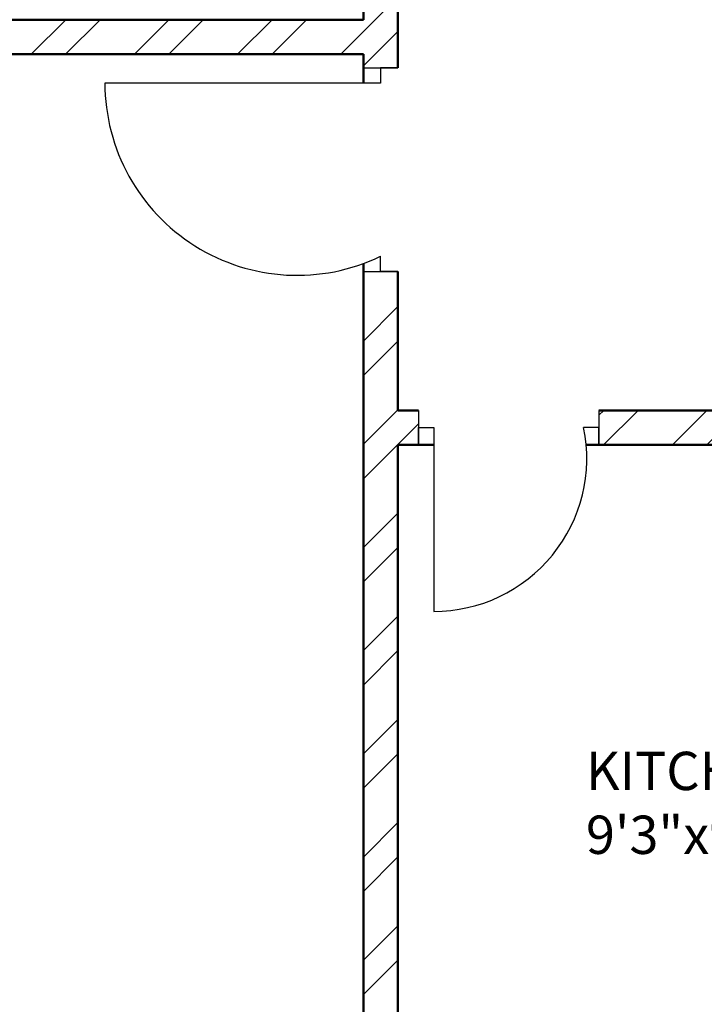
# Model space of a CAD drawing. Units: inches. Extents: x 963 to 2075, y 289 to 2657.
# Tile 44 of 98: x 1600 to 1689, y 1585 to 1714. Entities that reach past the tile are written whole.
import ezdxf

# ---------------------------------------------------------------- set-up
doc = ezdxf.new("R2010")
doc.units = ezdxf.units.IN
for name, color, linetype, lineweight in [('A-AREA-IDEN', 7, 'Continuous', 18), ('A-DOOR', 4, 'Continuous', 25), ('A-WALL', 7, 'Continuous', 50), ('A-WALL-PATT', 8, 'Continuous', 13)]:
    doc.layers.add(name, color=color, linetype=linetype, lineweight=lineweight)
doc.styles.get("Standard").update_dxf_attribs({"font": 'arial.ttf'})

msp = doc.modelspace()

# ---------------------------------------------------------------- hatches: boundary and pattern name
at = {"layer": 'A-WALL-PATT'}
h = msp.add_hatch(dxfattribs=at)
h.set_pattern_fill('ANSI32', color=256)
h.paths.add_polyline_path([(1296.92, 2558.32), (1203.92, 2558.32), (1203.92, 2493.82), (1191.53, 2493.82), (1191.53, 2489.32), (1211.06, 2489.32), (1211.06, 2492.02), (1211.06, 2493.82), (1208.42, 2493.82), (1208.42, 2553.82), (1292.42, 2553.82), (1292.42, 2538.86), (1296.92, 2538.86)])
h.paths.add_polyline_path([(1442.42, 2558.32), (1349.42, 2558.32), (1349.42, 2538.94), (1353.92, 2538.94), (1353.92, 2553.82), (1437.92, 2553.82), (1437.92, 2493.82), (1434.54, 2493.82), (1434.54, 2489.32), (1448.31, 2489.32), (1448.31, 2491.57), (1448.31, 2493.82), (1442.42, 2493.82)])
h.paths.add_polyline_path([(1415.55, 2491.57), (1415.55, 2493.82), (1340.94, 2493.82), (1340.94, 2489.32), (1371.92, 2489.32), (1371.92, 2378.32), (1367.6, 2378.32), (1367.6, 2373.82), (1371.92, 2373.82), (1371.92, 2355.19), (1376.42, 2355.19), (1376.42, 2489.32), (1415.55, 2489.32)])
h.paths.add_polyline_path([(1304.94, 2491.57), (1304.94, 2493.82), (1296.92, 2493.82), (1296.92, 2514.86), (1292.42, 2514.86), (1292.42, 2493.82), (1232.81, 2493.82), (1232.81, 2489.32), (1256.42, 2489.32), (1256.42, 2327.32), (1253.71, 2327.32), (1253.71, 2322.82), (1328.42, 2322.82), (1328.42, 2331.15), (1323.92, 2331.15), (1323.92, 2327.32), (1260.92, 2327.32), (1260.92, 2373.82), (1323.92, 2373.82), (1323.92, 2357.81), (1328.42, 2357.81), (1328.42, 2373.82), (1346.01, 2373.82), (1346.01, 2376.07), (1346.01, 2378.32), (1260.92, 2378.32), (1260.92, 2489.32), (1304.94, 2489.32)])
h.paths.add_polyline_path([(1226.65, 2327.32), (1124.42, 2327.32), (1124.42, 2347.45), (1119.92, 2347.45), (1119.92, 2322.82), (1163.42, 2322.82), (1163.42, 2305.43), (1165.67, 2305.43), (1167.92, 2305.43), (1167.92, 2322.82), (1226.65, 2322.82), (1226.65, 2325.07)])
h.paths.add_polyline_path([(1095.92, 2489.32), (1124.42, 2489.32), (1131.53, 2489.32), (1131.53, 2491.57), (1131.53, 2493.82), (1119.92, 2493.82), (1091.42, 2493.82), (1091.42, 2417.32), (1095.92, 2417.32), (1119.92, 2417.32), (1119.92, 2407.45), (1124.42, 2407.45), (1124.42, 2421.82), (1095.92, 2421.82)])
h.paths.add_polyline_path([(1512.92, 2558.32), (1508.42, 2558.32), (1508.42, 2493.82), (1503.4, 2493.82), (1503.4, 2489.32), (1508.42, 2489.32), (1508.42, 2327.32), (1376.42, 2327.32), (1376.42, 2330.27), (1371.92, 2330.27), (1371.92, 2298.74), (1376.42, 2298.74), (1376.42, 2322.82), (1508.42, 2322.82), (1508.42, 2165.32), (1504.26, 2165.32), (1504.26, 2160.82), (1508.42, 2160.82), (1508.42, 2108.32), (1512.92, 2108.32), (1512.92, 2160.82), (1516.18, 2160.82), (1516.18, 2163.07), (1516.18, 2165.32), (1512.92, 2165.32), (1512.92, 2322.82), (1644.92, 2322.82), (1644.92, 2298.74), (1649.42, 2298.74), (1649.42, 2322.82), (1649.42, 2330.94), (1647.17, 2330.94), (1644.92, 2330.94), (1644.92, 2327.32), (1512.92, 2327.32), (1512.92, 2489.32), (1516.76, 2489.32), (1516.76, 2491.57), (1516.76, 2493.82), (1512.92, 2493.82)])
h.paths.add_polyline_path([(1671.92, 2558.32), (1578.92, 2558.32), (1578.92, 2493.82), (1573.53, 2493.82), (1573.53, 2489.32), (1586.54, 2489.32), (1586.54, 2491.57), (1586.54, 2493.82), (1583.42, 2493.82), (1583.42, 2553.82), (1667.42, 2553.82), (1667.42, 2541.11), (1671.92, 2541.11)])
h.paths.add_polyline_path([(1681.26, 2493.82), (1671.92, 2493.82), (1671.92, 2517.11), (1667.42, 2517.11), (1667.42, 2493.82), (1610.22, 2493.82), (1610.22, 2489.32), (1644.92, 2489.32), (1644.92, 2357.87), (1649.42, 2357.87), (1649.42, 2373.82), (1652.2, 2373.82), (1652.2, 2375.83), (1652.2, 2378.32), (1649.42, 2378.32), (1649.42, 2489.32), (1681.26, 2489.32), (1681.26, 2491.57)])
h.paths.add_polyline_path([(1821.92, 2558.32), (1728.92, 2558.32), (1728.92, 2541), (1733.42, 2541), (1733.42, 2553.82), (1817.42, 2553.82), (1817.42, 2493.82), (1813.51, 2493.82), (1813.51, 2489.32), (1830.08, 2489.32), (1830.08, 2491.57), (1830.08, 2493.82), (1821.92, 2493.82)])
h.paths.add_polyline_path([(1794.24, 2493.82), (1717.26, 2493.82), (1717.26, 2489.32), (1760.42, 2489.32), (1760.42, 2378.32), (1674.4, 2378.32), (1674.4, 2373.82), (1692.92, 2373.82), (1692.92, 2356.95), (1697.42, 2356.95), (1697.42, 2373.82), (1760.42, 2373.82), (1760.42, 2327.32), (1697.42, 2327.32), (1697.42, 2333.34), (1692.92, 2333.34), (1692.92, 2322.82), (1768.04, 2322.82), (1768.04, 2325.07), (1768.04, 2327.32), (1764.92, 2327.32), (1764.92, 2489.32), (1794.24, 2489.32)])
h.paths.add_polyline_path([(1733.42, 2517), (1728.92, 2517), (1728.92, 2493.82), (1733.42, 2493.82)], flags=17)
h.paths.add_polyline_path([(1929.92, 2493.82), (1890.08, 2493.82), (1890.08, 2489.32), (1896.92, 2489.32), (1925.42, 2489.32), (1925.42, 2421.82), (1896.92, 2421.82), (1896.92, 2408.32), (1901.42, 2408.32), (1901.42, 2417.32), (1925.42, 2417.32), (1929.92, 2417.32)])
h.paths.add_polyline_path([(1901.42, 2348.32), (1896.92, 2348.32), (1896.92, 2327.32), (1800.42, 2327.32), (1800.42, 2322.82), (1853.42, 2322.82), (1853.42, 2309.45), (1857.92, 2309.45), (1857.92, 2322.82), (1901.42, 2322.82)])
h.paths.add_polyline_path([(1857.92, 2249.45), (1853.42, 2249.45), (1853.42, 2214.82), (1686.31, 2214.82), (1686.31, 2210.32), (1853.42, 2210.32), (1853.42, 2202.13), (1857.92, 2202.13), (1857.92, 2210.32)])
h.paths.add_polyline_path([(1857.92, 2142.13), (1853.42, 2142.13), (1853.42, 2115.42), (1841.42, 2115.42), (1841.42, 2088.53), (1841.42, 2046.95), (1845.92, 2046.95), (1845.92, 2110.92), (1905.92, 2110.92), (1905.92, 2092.52), (1910.42, 2092.52), (1910.42, 2115.42), (1857.92, 2115.42)])
h.paths.add_polyline_path([(1532.44, 1482.34), (1573.46, 1482.34), (1573.46, 1501), (1532.44, 1501)], flags=9)
h.paths.add_polyline_path([(1438.66, 1486.3), (1479.68, 1486.3), (1479.68, 1504.96), (1438.66, 1504.96)], flags=9)
h.paths.add_polyline_path([(1411.22, 1365.31), (1659.14, 1365.31), (1659.14, 1402.4), (1411.22, 1402.4)], flags=9)
h.paths.add_polyline_path([(1185.67, 2296.3), (1248.16, 2296.3), (1248.16, 2314.95), (1185.67, 2314.95)], flags=9)
h.paths.add_polyline_path([(1177.31, 2187.35), (1216.15, 2187.35), (1216.15, 2206.01), (1177.31, 2206.01)], flags=9)
h.paths.add_polyline_path([(1295.1, 1602.08), (1328.26, 1602.08), (1328.26, 1620.74), (1295.1, 1620.74)], flags=9)
h.paths.add_polyline_path([(1525.13, 2005.99), (1558.39, 2005.99), (1558.39, 2024.65), (1525.13, 2024.65)], flags=9)
h.paths.add_polyline_path([(1459.61, 1977.13), (1472.19, 1977.13), (1472.19, 1987.43), (1459.61, 1987.43)], flags=9)
h.paths.add_polyline_path([(1467.81, 2053.68), (1480.02, 2053.68), (1480.02, 2063.98), (1467.81, 2063.98)], flags=9)
h.paths.add_polyline_path([(1555.18, 2119.02), (1584.56, 2119.02), (1584.56, 2137.68), (1555.18, 2137.68)], flags=25)
h.paths.add_polyline_path([(1405.39, 2115.29), (1444.48, 2115.29), (1444.48, 2133.95), (1405.39, 2133.95)], flags=25)
h.paths.add_polyline_path([(1698.48, 2004.26), (1727.69, 2004.26), (1727.69, 2022.92), (1698.48, 2022.92)], flags=9)
h.paths.add_polyline_path([(1612.16, 1972.86), (1629.02, 1972.86), (1629.02, 1983.16), (1612.16, 1983.16)], flags=9)
h.paths.add_polyline_path([(1608.29, 2060.04), (1625.15, 2060.04), (1625.15, 2070.34), (1608.29, 2070.34)], flags=9)
h.paths.add_polyline_path([(1527.95, 1684.4), (1566.79, 1684.4), (1566.79, 1703.06), (1527.95, 1703.06)], flags=9)
h.paths.add_polyline_path([(1422.79, 1683.59), (1461.63, 1683.59), (1461.63, 1702.25), (1422.79, 1702.25)], flags=9)
h.paths.add_polyline_path([(1531.26, 1732.46), (1574.01, 1732.46), (1574.01, 1751.12), (1531.26, 1751.12)], flags=9)
h.paths.add_polyline_path([(1402.87, 1732.85), (1439.8, 1732.85), (1439.8, 1751.5), (1402.87, 1751.5)], flags=9)
h.paths.add_polyline_path([(1243.12, 1923.13), (1281.96, 1923.13), (1281.96, 1941.79), (1243.12, 1941.79)], flags=9)
h.paths.add_polyline_path([(1181.75, 1792.27), (1244.24, 1792.27), (1244.24, 1810.93), (1181.75, 1810.93)], flags=9)
h.paths.add_polyline_path([(1265.82, 1670.3), (1316.07, 1670.3), (1316.07, 1688.96), (1265.82, 1688.96)], flags=9)
h.paths.add_polyline_path([(1140.26, 1676.05), (1179.1, 1676.05), (1179.1, 1694.71), (1140.26, 1694.71)], flags=9)
h.paths.add_polyline_path([(1107.49, 1490.89), (1143.37, 1490.89), (1143.37, 1509.55), (1107.49, 1509.55)], flags=9)
h.paths.add_polyline_path([(1217.58, 1483.9), (1246.74, 1483.9), (1246.74, 1502.56), (1217.58, 1502.56)], flags=9)
h.paths.add_polyline_path([(1389.21, 1486.92), (1418.37, 1486.92), (1418.37, 1505.58), (1389.21, 1505.58)], flags=9)
h.paths.add_polyline_path([(1672.21, 1602.08), (1705.37, 1602.08), (1705.37, 1620.74), (1672.21, 1620.74)], flags=9)
h.paths.add_polyline_path([(1752.08, 1522.64), (1781.24, 1522.64), (1781.24, 1541.3), (1752.08, 1541.3)], flags=9)
h.paths.add_polyline_path([(1848.27, 1491.26), (1884.16, 1491.26), (1884.16, 1509.92), (1848.27, 1509.92)], flags=9)
h.paths.add_polyline_path([(1822.47, 1685.62), (1861.31, 1685.62), (1861.31, 1704.28), (1822.47, 1704.28)], flags=9)
h.paths.add_polyline_path([(1713.19, 1672.23), (1763.44, 1672.23), (1763.44, 1690.89), (1713.19, 1690.89)], flags=9)
h.paths.add_polyline_path([(1736.62, 1790.58), (1799.11, 1790.58), (1799.11, 1809.24), (1736.62, 1809.24)], flags=9)
h.paths.add_polyline_path([(1691.49, 1916.36), (1730.33, 1916.36), (1730.33, 1935.01), (1691.49, 1935.01)], flags=9)
h.paths.add_polyline_path([(1764.87, 1973.92), (1794.31, 1973.92), (1794.31, 1992.58), (1764.87, 1992.58)], flags=9)
h.paths.add_polyline_path([(1767.85, 2034.02), (1797.29, 2034.02), (1797.29, 2052.67), (1767.85, 2052.67)], flags=9)
h.paths.add_polyline_path([(1851.59, 2060.33), (1880.75, 2060.33), (1880.75, 2078.99), (1851.59, 2078.99)], flags=25)
h.paths.add_polyline_path([(1688.49, 2086.87), (1727.33, 2086.87), (1727.33, 2105.53), (1688.49, 2105.53)], flags=9)
h.paths.add_polyline_path([(1537.74, 2293.58), (1580.49, 2293.58), (1580.49, 2312.24), (1537.74, 2312.24)], flags=25)
h.paths.add_polyline_path([(1425.59, 2296.11), (1468.34, 2296.11), (1468.34, 2314.77), (1425.59, 2314.77)], flags=25)
h.paths.add_polyline_path([(1278.52, 2004.18), (1307.72, 2004.18), (1307.72, 2022.84), (1278.52, 2022.84)], flags=9)
h.paths.add_polyline_path([(1193.28, 1973.63), (1222.72, 1973.63), (1222.72, 1992.29), (1193.28, 1992.29)], flags=9)
h.paths.add_polyline_path([(1192.41, 2040.58), (1221.84, 2040.58), (1221.84, 2059.23), (1192.41, 2059.23)], flags=9)
h.paths.add_polyline_path([(1130.6, 1951.39), (1159.76, 1951.39), (1159.76, 1970.05), (1130.6, 1970.05)], flags=9)
h.paths.add_polyline_path([(1132.83, 2052.49), (1161.98, 2052.49), (1161.98, 2071.15), (1132.83, 2071.15)], flags=9)
h.paths.add_polyline_path([(1265.13, 2334.62), (1315.38, 2334.62), (1315.38, 2353.28), (1265.13, 2353.28)], flags=25)
h.paths.add_polyline_path([(1136.74, 2330.79), (1175.58, 2330.79), (1175.58, 2349.44), (1136.74, 2349.44)], flags=9)
h.paths.add_polyline_path([(1287.42, 2417.2), (1320.58, 2417.2), (1320.58, 2435.86), (1287.42, 2435.86)], flags=25)
h.paths.add_polyline_path([(1430.99, 2329.16), (1469.83, 2329.16), (1469.83, 2347.82), (1430.99, 2347.82)], flags=25)
h.paths.add_polyline_path([(1525.42, 2329.21), (1564.26, 2329.21), (1564.26, 2347.87), (1525.42, 2347.87)], flags=25)
h.paths.add_polyline_path([(1684.52, 2382.8), (1717.68, 2382.8), (1717.68, 2401.46), (1684.52, 2401.46)], flags=25)
h.paths.add_polyline_path([(1704.81, 2340.29), (1755.05, 2340.29), (1755.05, 2358.95), (1704.81, 2358.95)], flags=25)
h.paths.add_polyline_path([(1694.11, 2287.76), (1756.6, 2287.76), (1756.6, 2306.41), (1694.11, 2306.41)], flags=9)
h.paths.add_polyline_path([(1815.78, 2329.86), (1854.62, 2329.86), (1854.62, 2348.52), (1815.78, 2348.52)], flags=9)
h.paths.add_polyline_path([(1842.87, 2514.26), (1878.76, 2514.26), (1878.76, 2532.91), (1842.87, 2532.91)], flags=9)
h.paths.add_polyline_path([(1769.51, 2531.45), (1798.67, 2531.45), (1798.67, 2550.1), (1769.51, 2550.1)], flags=25)
h.paths.add_polyline_path([(1594.77, 2518.47), (1623.93, 2518.47), (1623.93, 2537.13), (1594.77, 2537.13)], flags=25)
h.paths.add_polyline_path([(1520.72, 2516.18), (1556.61, 2516.18), (1556.61, 2534.84), (1520.72, 2534.84)], flags=25)
h.paths.add_polyline_path([(1464.46, 2516.69), (1500.34, 2516.69), (1500.34, 2535.35), (1464.46, 2535.35)], flags=25)
h.paths.add_polyline_path([(1365.7, 2528.97), (1394.85, 2528.97), (1394.85, 2547.63), (1365.7, 2547.63)], flags=25)
h.paths.add_polyline_path([(1222.84, 2516.23), (1252, 2516.23), (1252, 2534.89), (1222.84, 2534.89)], flags=25)
h.paths.add_polyline_path([(1104.55, 2509.6), (1140.43, 2509.6), (1140.43, 2528.26), (1104.55, 2528.26)], flags=9)
h = msp.add_hatch(dxfattribs=at)
h.set_pattern_fill('ANSI32', color=256)
h.paths.add_polyline_path([(1335.97, 2212.57), (1335.97, 2214.82), (1167.92, 2214.82), (1167.92, 2245.43), (1163.42, 2245.43), (1163.42, 2210.32), (1163.42, 2194.81), (1167.92, 2194.81), (1167.92, 2210.32), (1335.97, 2210.32)])
h.paths.add_polyline_path([(1532.44, 1482.34), (1573.46, 1482.34), (1573.46, 1501), (1532.44, 1501)], flags=9)
h.paths.add_polyline_path([(1438.66, 1486.3), (1479.68, 1486.3), (1479.68, 1504.96), (1438.66, 1504.96)], flags=9)
h.paths.add_polyline_path([(1411.22, 1365.31), (1659.14, 1365.31), (1659.14, 1402.4), (1411.22, 1402.4)], flags=9)
h.paths.add_polyline_path([(1185.67, 2296.3), (1248.16, 2296.3), (1248.16, 2314.95), (1185.67, 2314.95)], flags=9)
h.paths.add_polyline_path([(1177.31, 2187.35), (1216.15, 2187.35), (1216.15, 2206.01), (1177.31, 2206.01)], flags=9)
h.paths.add_polyline_path([(1295.1, 1602.08), (1328.26, 1602.08), (1328.26, 1620.74), (1295.1, 1620.74)], flags=9)
h.paths.add_polyline_path([(1525.13, 2005.99), (1558.39, 2005.99), (1558.39, 2024.65), (1525.13, 2024.65)], flags=9)
h.paths.add_polyline_path([(1459.61, 1977.13), (1472.19, 1977.13), (1472.19, 1987.43), (1459.61, 1987.43)], flags=9)
h.paths.add_polyline_path([(1467.81, 2053.68), (1480.02, 2053.68), (1480.02, 2063.98), (1467.81, 2063.98)], flags=9)
h.paths.add_polyline_path([(1555.18, 2119.02), (1584.56, 2119.02), (1584.56, 2137.68), (1555.18, 2137.68)], flags=9)
h.paths.add_polyline_path([(1405.39, 2115.29), (1444.48, 2115.29), (1444.48, 2133.95), (1405.39, 2133.95)], flags=9)
h.paths.add_polyline_path([(1698.48, 2004.26), (1727.69, 2004.26), (1727.69, 2022.92), (1698.48, 2022.92)], flags=9)
h.paths.add_polyline_path([(1612.16, 1972.86), (1629.02, 1972.86), (1629.02, 1983.16), (1612.16, 1983.16)], flags=9)
h.paths.add_polyline_path([(1608.29, 2060.04), (1625.15, 2060.04), (1625.15, 2070.34), (1608.29, 2070.34)], flags=9)
h.paths.add_polyline_path([(1527.95, 1684.4), (1566.79, 1684.4), (1566.79, 1703.06), (1527.95, 1703.06)], flags=9)
h.paths.add_polyline_path([(1422.79, 1683.59), (1461.63, 1683.59), (1461.63, 1702.25), (1422.79, 1702.25)], flags=9)
h.paths.add_polyline_path([(1531.26, 1732.46), (1574.01, 1732.46), (1574.01, 1751.12), (1531.26, 1751.12)], flags=9)
h.paths.add_polyline_path([(1402.87, 1732.85), (1439.8, 1732.85), (1439.8, 1751.5), (1402.87, 1751.5)], flags=9)
h.paths.add_polyline_path([(1243.12, 1923.13), (1281.96, 1923.13), (1281.96, 1941.79), (1243.12, 1941.79)], flags=9)
h.paths.add_polyline_path([(1181.75, 1792.27), (1244.24, 1792.27), (1244.24, 1810.93), (1181.75, 1810.93)], flags=9)
h.paths.add_polyline_path([(1265.82, 1670.3), (1316.07, 1670.3), (1316.07, 1688.96), (1265.82, 1688.96)], flags=9)
h.paths.add_polyline_path([(1140.26, 1676.05), (1179.1, 1676.05), (1179.1, 1694.71), (1140.26, 1694.71)], flags=9)
h.paths.add_polyline_path([(1107.49, 1490.89), (1143.37, 1490.89), (1143.37, 1509.55), (1107.49, 1509.55)], flags=9)
h.paths.add_polyline_path([(1217.58, 1483.9), (1246.74, 1483.9), (1246.74, 1502.56), (1217.58, 1502.56)], flags=9)
h.paths.add_polyline_path([(1389.21, 1486.92), (1418.37, 1486.92), (1418.37, 1505.58), (1389.21, 1505.58)], flags=9)
h.paths.add_polyline_path([(1672.21, 1602.08), (1705.37, 1602.08), (1705.37, 1620.74), (1672.21, 1620.74)], flags=9)
h.paths.add_polyline_path([(1752.08, 1522.64), (1781.24, 1522.64), (1781.24, 1541.3), (1752.08, 1541.3)], flags=9)
h.paths.add_polyline_path([(1848.27, 1491.26), (1884.16, 1491.26), (1884.16, 1509.92), (1848.27, 1509.92)], flags=9)
h.paths.add_polyline_path([(1822.47, 1685.62), (1861.31, 1685.62), (1861.31, 1704.28), (1822.47, 1704.28)], flags=9)
h.paths.add_polyline_path([(1713.19, 1672.23), (1763.44, 1672.23), (1763.44, 1690.89), (1713.19, 1690.89)], flags=9)
h.paths.add_polyline_path([(1736.62, 1790.58), (1799.11, 1790.58), (1799.11, 1809.24), (1736.62, 1809.24)], flags=9)
h.paths.add_polyline_path([(1691.49, 1916.36), (1730.33, 1916.36), (1730.33, 1935.01), (1691.49, 1935.01)], flags=9)
h.paths.add_polyline_path([(1764.87, 1973.92), (1794.31, 1973.92), (1794.31, 1992.58), (1764.87, 1992.58)], flags=9)
h.paths.add_polyline_path([(1767.85, 2034.02), (1797.29, 2034.02), (1797.29, 2052.67), (1767.85, 2052.67)], flags=9)
h.paths.add_polyline_path([(1851.59, 2060.33), (1880.75, 2060.33), (1880.75, 2078.99), (1851.59, 2078.99)], flags=9)
h.paths.add_polyline_path([(1688.49, 2086.87), (1727.33, 2086.87), (1727.33, 2105.53), (1688.49, 2105.53)], flags=9)
h.paths.add_polyline_path([(1537.74, 2293.58), (1580.49, 2293.58), (1580.49, 2312.24), (1537.74, 2312.24)], flags=9)
h.paths.add_polyline_path([(1425.59, 2296.11), (1468.34, 2296.11), (1468.34, 2314.77), (1425.59, 2314.77)], flags=9)
h.paths.add_polyline_path([(1278.52, 2004.18), (1307.72, 2004.18), (1307.72, 2022.84), (1278.52, 2022.84)], flags=9)
h.paths.add_polyline_path([(1193.28, 1973.63), (1222.72, 1973.63), (1222.72, 1992.29), (1193.28, 1992.29)], flags=9)
h.paths.add_polyline_path([(1192.41, 2040.58), (1221.84, 2040.58), (1221.84, 2059.23), (1192.41, 2059.23)], flags=9)
h.paths.add_polyline_path([(1130.6, 1951.39), (1159.76, 1951.39), (1159.76, 1970.05), (1130.6, 1970.05)], flags=9)
h.paths.add_polyline_path([(1132.83, 2052.49), (1161.98, 2052.49), (1161.98, 2071.15), (1132.83, 2071.15)], flags=9)
h.paths.add_polyline_path([(1265.13, 2334.62), (1315.38, 2334.62), (1315.38, 2353.28), (1265.13, 2353.28)], flags=9)
h.paths.add_polyline_path([(1136.74, 2330.79), (1175.58, 2330.79), (1175.58, 2349.44), (1136.74, 2349.44)], flags=9)
h.paths.add_polyline_path([(1287.42, 2417.2), (1320.58, 2417.2), (1320.58, 2435.86), (1287.42, 2435.86)], flags=9)
h.paths.add_polyline_path([(1430.99, 2329.16), (1469.83, 2329.16), (1469.83, 2347.82), (1430.99, 2347.82)], flags=9)
h.paths.add_polyline_path([(1525.42, 2329.21), (1564.26, 2329.21), (1564.26, 2347.87), (1525.42, 2347.87)], flags=9)
h.paths.add_polyline_path([(1684.52, 2382.8), (1717.68, 2382.8), (1717.68, 2401.46), (1684.52, 2401.46)], flags=9)
h.paths.add_polyline_path([(1704.81, 2340.29), (1755.05, 2340.29), (1755.05, 2358.95), (1704.81, 2358.95)], flags=9)
h.paths.add_polyline_path([(1694.11, 2287.76), (1756.6, 2287.76), (1756.6, 2306.41), (1694.11, 2306.41)], flags=9)
h.paths.add_polyline_path([(1815.78, 2329.86), (1854.62, 2329.86), (1854.62, 2348.52), (1815.78, 2348.52)], flags=9)
h.paths.add_polyline_path([(1842.87, 2514.26), (1878.76, 2514.26), (1878.76, 2532.91), (1842.87, 2532.91)], flags=9)
h.paths.add_polyline_path([(1769.51, 2531.45), (1798.67, 2531.45), (1798.67, 2550.1), (1769.51, 2550.1)], flags=9)
h.paths.add_polyline_path([(1594.77, 2518.47), (1623.93, 2518.47), (1623.93, 2537.13), (1594.77, 2537.13)], flags=9)
h.paths.add_polyline_path([(1520.72, 2516.18), (1556.61, 2516.18), (1556.61, 2534.84), (1520.72, 2534.84)], flags=9)
h.paths.add_polyline_path([(1464.46, 2516.69), (1500.34, 2516.69), (1500.34, 2535.35), (1464.46, 2535.35)], flags=9)
h.paths.add_polyline_path([(1365.7, 2528.97), (1394.85, 2528.97), (1394.85, 2547.63), (1365.7, 2547.63)], flags=9)
h.paths.add_polyline_path([(1222.84, 2516.23), (1252, 2516.23), (1252, 2534.89), (1222.84, 2534.89)], flags=9)
h.paths.add_polyline_path([(1104.55, 2509.6), (1140.43, 2509.6), (1140.43, 2528.26), (1104.55, 2528.26)], flags=9)
h = msp.add_hatch(dxfattribs=at)
h.set_pattern_fill('ANSI32', color=256)
h.paths.add_polyline_path([(1473.61, 2163.07), (1473.61, 2165.32), (1376.42, 2165.32), (1376.42, 2227.98), (1371.92, 2227.98), (1371.92, 2214.82), (1368.41, 2214.82), (1368.41, 2210.32), (1371.92, 2210.32), (1371.92, 2160.82), (1395.92, 2160.82), (1395.92, 2090.32), (1217.34, 2090.32), (1217.34, 2085.82), (1395.92, 2085.82), (1458.92, 2085.82), (1458.92, 2108.32), (1454.42, 2108.32), (1454.42, 2090.32), (1400.42, 2090.32), (1400.42, 2160.82), (1473.61, 2160.82)])
h.paths.add_polyline_path([(1649.42, 2210.32), (1653.23, 2210.32), (1653.23, 2214.82), (1649.42, 2214.82), (1649.42, 2227.98), (1644.92, 2227.98), (1644.92, 2165.32), (1550.1, 2165.32), (1550.1, 2160.82), (1620.92, 2160.82), (1620.92, 2112.82), (1555.45, 2112.82), (1555.45, 2108.32), (1584.33, 2108.32), (1584.33, 2084.92), (1588.83, 2084.92), (1588.83, 2108.32), (1625.42, 2108.32), (1667.95, 2108.32), (1667.95, 2022.67), (1588.83, 2022.67), (1588.83, 2047.41), (1584.33, 2047.41), (1584.33, 1996), (1588.83, 1996), (1588.83, 2018.32), (1667.95, 2018.17), (1667.95, 1928.32), (1625.42, 1928.32), (1625.42, 1923.82), (1672.45, 1923.82), (1672.45, 1928.32), (1672.45, 1946.66), (1785.45, 1946.66), (1785.45, 1951.16), (1743.03, 1951.16), (1743.03, 2017.92), (1841.42, 2017.92), (1841.42, 2014.77), (1845.92, 2014.77), (1845.92, 2017.92), (1905.92, 2017.92), (1905.92, 1987.51), (1910.42, 1987.51), (1910.42, 2022.42), (1910.42, 2068.52), (1905.92, 2068.52), (1905.92, 2022.42), (1845.92, 2022.42), (1845.92, 2025.85), (1843.67, 2025.85), (1841.42, 2025.85), (1841.42, 2022.42), (1743.03, 2022.42), (1743.03, 2084.03), (1768.45, 2084.03), (1785.45, 2084.03), (1785.45, 2088.53), (1672.45, 2088.53), (1672.45, 2112.82), (1667.95, 2112.82), (1625.42, 2112.82), (1625.42, 2160.82), (1649.42, 2160.82)])
h.paths.add_polyline_path([(1672.45, 2084.03), (1738.53, 2084.03), (1738.53, 1951.16), (1672.45, 1951.16)], flags=16)
h.paths.add_polyline_path([(1672.45, 2084.03), (1738.53, 2084.03), (1705.49, 2017.6)], flags=0)
h.paths.add_polyline_path([(1262.77, 2085.82), (1258.27, 2085.82), (1258.27, 2023.28), (1184.42, 2023.28), (1184.42, 2018.78), (1258.27, 2018.78), (1258.27, 1950.82), (1262.77, 1950.82)])
h.paths.add_polyline_path([(1312.27, 2085.82), (1307.77, 2085.82), (1307.77, 1950.82), (1312.27, 1950.82)])
h.paths.add_polyline_path([(1458.92, 1950.82), (1395.92, 1950.82), (1216.57, 1950.82), (1216.57, 1946.32), (1346.42, 1946.32), (1395.92, 1946.32), (1395.92, 1875.82), (1371.92, 1875.82), (1371.92, 1826.32), (1368.93, 1826.32), (1368.93, 1821.82), (1371.92, 1821.82), (1371.92, 1813.62), (1376.42, 1813.62), (1376.42, 1871.32), (1474.5, 1871.32), (1474.5, 1873.57), (1474.5, 1875.82), (1400.42, 1875.82), (1400.42, 1946.32), (1454.42, 1946.32), (1454.42, 1928.32), (1458.92, 1928.32)])
h.paths.add_polyline_path([(1184.42, 2120.78), (1167.92, 2120.78), (1167.92, 2134.81), (1165.67, 2134.81), (1163.42, 2134.81), (1163.42, 2120.78), (1119.92, 2120.78), (1119.92, 2098.1), (1124.42, 2098.1), (1124.42, 2116.28), (1167.92, 2116.28), (1179.92, 2116.28), (1179.92, 2045.92), (1184.42, 2045.92), (1184.42, 2090.32), (1184.42, 2116.28)])
h.paths.add_polyline_path([(1124.42, 2018.78), (1179.92, 2018.78), (1179.92, 2016.29), (1184.42, 2016.29), (1184.42, 2023.28), (1184.42, 2026.59), (1182.17, 2026.59), (1179.92, 2026.59), (1179.92, 2023.28), (1124.42, 2023.28), (1124.42, 2074.1), (1119.92, 2074.1), (1119.92, 2018.78), (1119.92, 1979.63), (1124.42, 1979.63)])
h.paths.add_polyline_path([(1184.42, 1925.78), (1184.42, 1946.32), (1184.42, 1996.07), (1182.17, 1996.07), (1179.92, 1996.07), (1179.92, 1925.78), (1124.42, 1925.78), (1124.42, 1955.63), (1119.92, 1955.5), (1119.92, 1921.28), (1158.92, 1921.28), (1158.92, 1909.98), (1163.42, 1909.98), (1163.42, 1921.28), (1184.42, 1921.28)])
h.paths.add_polyline_path([(1341.45, 1826.32), (1163.42, 1826.32), (1163.42, 1849.98), (1158.92, 1849.98), (1158.92, 1821.82), (1158.92, 1804.03), (1163.42, 1804.03), (1163.42, 1821.82), (1341.45, 1821.82)])
h.paths.add_polyline_path([(1222.98, 1713.82), (1163.42, 1713.82), (1163.42, 1744.03), (1161.17, 1744.03), (1158.92, 1744.03), (1158.92, 1713.82), (1119.92, 1713.82), (1119.92, 1694.65), (1124.42, 1694.65), (1124.42, 1709.32), (1158.92, 1709.32), (1222.98, 1709.32)])
h.paths.add_polyline_path([(1328.42, 1713.82), (1252.04, 1713.82), (1252.04, 1711.57), (1252.04, 1709.32), (1256.42, 1709.32), (1256.42, 1547.32), (1232.94, 1547.32), (1232.94, 1545.07), (1232.94, 1542.82), (1292.42, 1542.82), (1292.42, 1527.63), (1296.92, 1527.63), (1296.92, 1542.82), (1299.46, 1542.82), (1299.46, 1547.32), (1260.92, 1547.32), (1260.92, 1658.32), (1343.66, 1658.32), (1343.66, 1660.57), (1343.66, 1662.82), (1328.42, 1662.82), (1328.42, 1676.59), (1327.4, 1676.59), (1323.92, 1676.59), (1323.92, 1662.82), (1260.92, 1662.82), (1260.92, 1709.32), (1323.92, 1709.32), (1323.92, 1699.85), (1328.42, 1699.85)])
h.paths.add_polyline_path([(1649.42, 1875.82), (1625.42, 1875.82), (1625.42, 1928.32), (1620.92, 1928.32), (1588.83, 1928.32), (1588.83, 1950.59), (1584.33, 1950.59), (1584.33, 1928.32), (1555.45, 1928.32), (1555.45, 1923.82), (1620.92, 1923.82), (1620.92, 1875.82), (1548.95, 1875.82), (1548.95, 1873.57), (1548.95, 1871.32), (1644.92, 1871.32), (1644.92, 1813.62), (1649.42, 1813.62), (1649.42, 1821.82), (1652.04, 1821.82), (1652.04, 1824.07), (1652.04, 1826.32), (1649.42, 1826.32)])
h.paths.add_polyline_path([(1512.92, 1871.32), (1516.48, 1871.32), (1516.48, 1875.82), (1512.92, 1875.82), (1512.92, 1923.82), (1512.92, 1928.32), (1512.92, 1930.83), (1508.42, 1930.83), (1508.42, 1875.82), (1504.41, 1875.82), (1504.41, 1871.32), (1508.42, 1871.32), (1508.42, 1713.82), (1376.42, 1713.82), (1376.42, 1743.32), (1371.92, 1743.32), (1371.92, 1709.32), (1371.92, 1706.01), (1376.42, 1706.01), (1376.42, 1709.32), (1508.42, 1709.32), (1508.42, 1547.32), (1501.87, 1547.32), (1501.87, 1542.82), (1508.42, 1542.82), (1508.42, 1482.82), (1508.42, 1436.32), (1512.92, 1436.32), (1512.92, 1542.82), (1519.32, 1542.82), (1519.32, 1545.07), (1519.32, 1547.32), (1512.92, 1547.32), (1512.92, 1709.32), (1644.92, 1709.32), (1644.92, 1707.55), (1649.42, 1707.55), (1649.42, 1709.32), (1649.42, 1743.32), (1644.92, 1743.32), (1644.92, 1713.82), (1512.92, 1713.82)])
h.paths.add_polyline_path([(1129.88, 1545.07), (1129.88, 1547.32), (1124.42, 1547.32), (1095.92, 1547.32), (1095.92, 1614.82), (1124.42, 1614.82), (1124.42, 1619.32), (1095.92, 1619.32), (1091.42, 1619.32), (1091.42, 1542.82), (1095.92, 1542.82), (1119.92, 1542.82), (1129.88, 1542.82)])
h.paths.add_polyline_path([(1208.42, 1542.82), (1211.74, 1542.82), (1211.74, 1547.32), (1198.85, 1547.32), (1198.85, 1542.82), (1203.92, 1542.82), (1203.92, 1478.32), (1208.42, 1478.32), (1296.92, 1478.32), (1296.92, 1503.63), (1292.42, 1503.63), (1292.42, 1482.82), (1208.42, 1482.82)])
h.paths.add_polyline_path([(1430.42, 1542.82), (1435.7, 1542.82), (1435.7, 1545.07), (1435.7, 1547.32), (1422.66, 1547.32), (1422.66, 1545.07), (1422.66, 1542.82), (1425.92, 1542.82), (1425.92, 1482.86), (1341.92, 1482.86), (1341.92, 1502.73), (1337.42, 1502.73), (1337.42, 1478.36), (1425.92, 1478.36), (1425.92, 1440.82), (1425.92, 1436.32), (1430.42, 1436.32)])
h.paths.add_polyline_path([(1698.48, 2004.26), (1727.69, 2004.26), (1727.69, 2022.92), (1698.48, 2022.92)], flags=8)
h = msp.add_hatch(dxfattribs=at)
h.set_pattern_fill('ANSI32', color=256)
h.paths.add_polyline_path([(1910.42, 1929.42), (1910.42, 1963.51), (1905.92, 1963.51), (1905.92, 1929.42), (1845.92, 1929.42), (1845.92, 1993.37), (1843.67, 1993.37), (1841.42, 1993.37), (1841.42, 1951.16), (1841.42, 1924.92), (1853.42, 1924.92), (1853.42, 1913.07), (1857.92, 1913.07), (1857.92, 1924.92), (1910.42, 1924.92)])
h.paths.add_polyline_path([(1857.92, 1853.07), (1853.42, 1853.07), (1853.42, 1826.32), (1841.42, 1826.32), (1674.48, 1826.32), (1674.48, 1821.82), (1853.42, 1821.82), (1857.92, 1821.82)])
h.paths.add_polyline_path([(1857.92, 1821.82), (1853.42, 1821.82), (1853.42, 1807.79), (1857.92, 1807.79)])
h.paths.add_polyline_path([(1857.92, 1747.79), (1853.42, 1747.79), (1853.42, 1713.82), (1809.34, 1713.82), (1809.34, 1709.32), (1905.92, 1709.32), (1905.92, 1688.32), (1910.42, 1688.32), (1910.42, 1713.82), (1857.92, 1713.82)])
h.paths.add_polyline_path([(1830.92, 1542.82), (1837.43, 1542.82), (1837.43, 1545.07), (1837.43, 1547.32), (1823.42, 1547.32), (1823.42, 1545.07), (1823.42, 1542.82), (1826.42, 1542.82), (1826.42, 1482.82), (1742.42, 1482.82), (1742.42, 1505.39), (1737.92, 1505.39), (1737.92, 1478.32), (1830.92, 1478.32)])
h.paths.add_polyline_path([(1938.92, 1619.32), (1934.42, 1619.32), (1910.42, 1619.32), (1910.42, 1628.32), (1908.17, 1628.32), (1905.92, 1628.32), (1905.92, 1614.82), (1934.42, 1614.82), (1934.42, 1547.32), (1905.92, 1547.32), (1899.59, 1547.32), (1899.59, 1542.82), (1910.42, 1542.82), (1938.92, 1542.82)])
h.paths.add_polyline_path([(1803.68, 1547.32), (1773.92, 1547.32), (1773.92, 1709.32), (1777.76, 1709.32), (1777.76, 1713.82), (1701.92, 1713.82), (1701.92, 1697.8), (1706.42, 1697.8), (1706.42, 1709.32), (1769.42, 1709.32), (1769.42, 1662.82), (1706.42, 1662.82), (1706.42, 1674.38), (1701.92, 1674.38), (1701.92, 1662.82), (1675.67, 1662.82), (1675.67, 1658.32), (1769.42, 1658.32), (1769.42, 1547.32), (1729.17, 1547.32), (1729.17, 1542.82), (1737.92, 1542.82), (1737.92, 1529.39), (1742.42, 1529.39), (1742.42, 1542.82), (1803.68, 1542.82)])
h.paths.add_polyline_path([(1595.42, 1542.82), (1599.24, 1542.82), (1599.24, 1547.32), (1584.36, 1547.32), (1584.36, 1542.82), (1590.92, 1542.82), (1590.92, 1436.32), (1595.42, 1436.32), (1595.42, 1440.82)])
h.paths.add_polyline_path([(1693.17, 1547.32), (1649.42, 1547.32), (1649.42, 1658.32), (1652.1, 1658.32), (1652.1, 1660.57), (1652.1, 1662.82), (1649.42, 1662.82), (1649.42, 1680.94), (1647.17, 1680.94), (1644.92, 1680.94), (1644.92, 1547.32), (1622.42, 1547.32), (1622.42, 1545.07), (1622.42, 1542.82), (1649.42, 1542.82), (1679.42, 1542.82), (1679.42, 1529.85), (1681.67, 1529.85), (1683.92, 1529.85), (1683.92, 1542.82), (1693.17, 1542.82), (1693.17, 1545.07)])
h.paths.add_polyline_path([(1683.92, 1505.85), (1679.42, 1505.85), (1679.42, 1483.8), (1595.42, 1483.8), (1595.42, 1479.3), (1683.92, 1479.3)])
h.paths.add_polyline_path([(1402.99, 1547.32), (1376.42, 1547.32), (1376.42, 1675.89), (1374.17, 1675.89), (1371.92, 1675.89), (1371.92, 1662.82), (1368.88, 1662.82), (1368.88, 1658.32), (1371.92, 1658.32), (1371.92, 1547.32), (1335.46, 1547.32), (1335.46, 1542.82), (1337.42, 1542.82), (1337.42, 1526.73), (1341.92, 1526.73), (1341.92, 1542.82), (1371.92, 1542.82), (1402.99, 1542.82)])

# ---------------------------------------------------------------- linework, layer by layer
at = {"layer": 'A-DOOR'}
for p, q in [((1644.92, 1707.55), (1649.42, 1707.55)), ((1649.42, 1707.55), (1647.17, 1707.55)), ((1647.17, 1707.55), (1647.17, 1705.55)), ((1647.17, 1705.55), (1611.17, 1705.55)), ((1647.17, 1680.94), (1647.17, 1682.94)), ((1644.92, 1680.94), (1649.42, 1680.94)), ((1649.42, 1680.94), (1647.17, 1680.94)), ((1652.1, 1662.82), (1652.1, 1658.32)), ((1675.67, 1662.82), (1675.67, 1658.32)), ((1652.1, 1658.32), (1652.1, 1660.57)), ((1652.1, 1660.57), (1654.1, 1660.57)), ((1654.1, 1660.57), (1654.1, 1636.57)), ((1675.67, 1660.57), (1673.67, 1660.57)), ((1675.67, 1658.32), (1675.67, 1660.57))]:
    msp.add_line(p, q, dxfattribs=at)
for centre, radius, start, end in [((1636.27, 1705.55), 25.1, 180, 295.7342), ((1654.1, 1656.55), 19.98, 270, 11.6004)]:
    msp.add_arc(centre, radius, start, end, dxfattribs=at)
at = {"layer": 'A-WALL'}
for p, q in [((1644.92, 1713.82), (1644.92, 1743.32)), ((1649.42, 1709.32), (1649.42, 1743.32)), ((1644.92, 1713.82), (1512.92, 1713.82)), ((1644.92, 1709.32), (1512.92, 1709.32)), ((1644.92, 1705.55), (1644.92, 1709.32)), ((1649.42, 1707.55), (1649.42, 1709.32)), ((1644.92, 1547.32), (1644.92, 1681.98)), ((1649.42, 1662.82), (1649.42, 1680.94)), ((1652.1, 1662.82), (1649.42, 1662.82)), ((1701.92, 1662.82), (1675.67, 1662.82)), ((1649.42, 1547.32), (1649.42, 1658.32)), ((1654.1, 1658.32), (1649.42, 1658.32)), ((1769.42, 1658.32), (1674, 1658.32))]:
    msp.add_line(p, q, dxfattribs=at)

# ---------------------------------------------------------------- texts
at = {"layer": 'A-AREA-IDEN', "insert": (1673.97, 1618.25), "char_height": 5, "attachment_point": 1}
msp.add_mtext_dynamic_manual_height_columns('KITCHEN\\P9\'3"x9\'3"', width=120.9099, gutter_width=12.5, heights=[0], dxfattribs=at)

doc.saveas('drawing.dxf')
